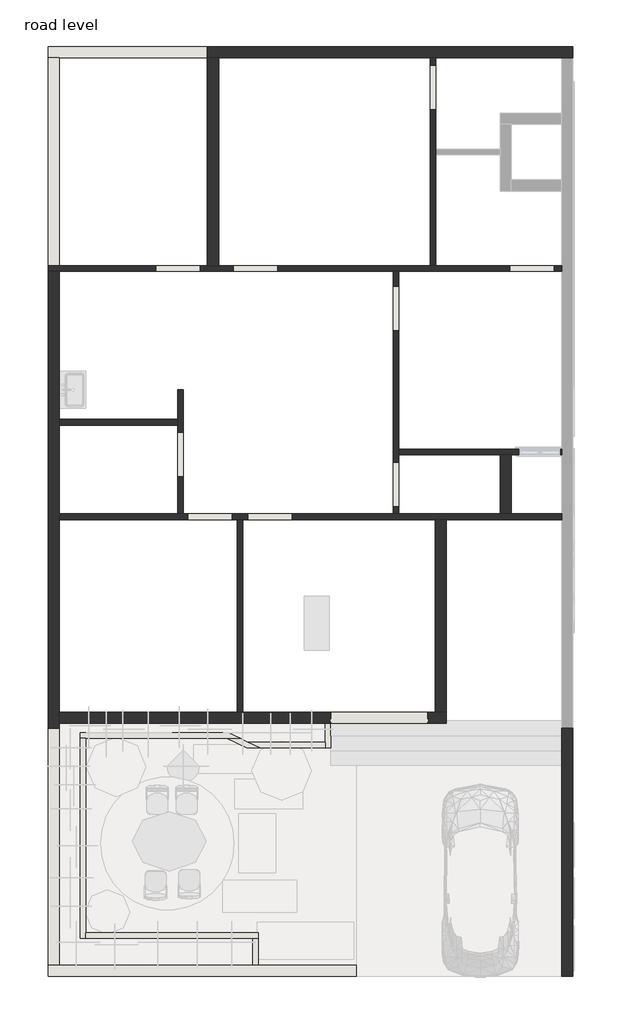
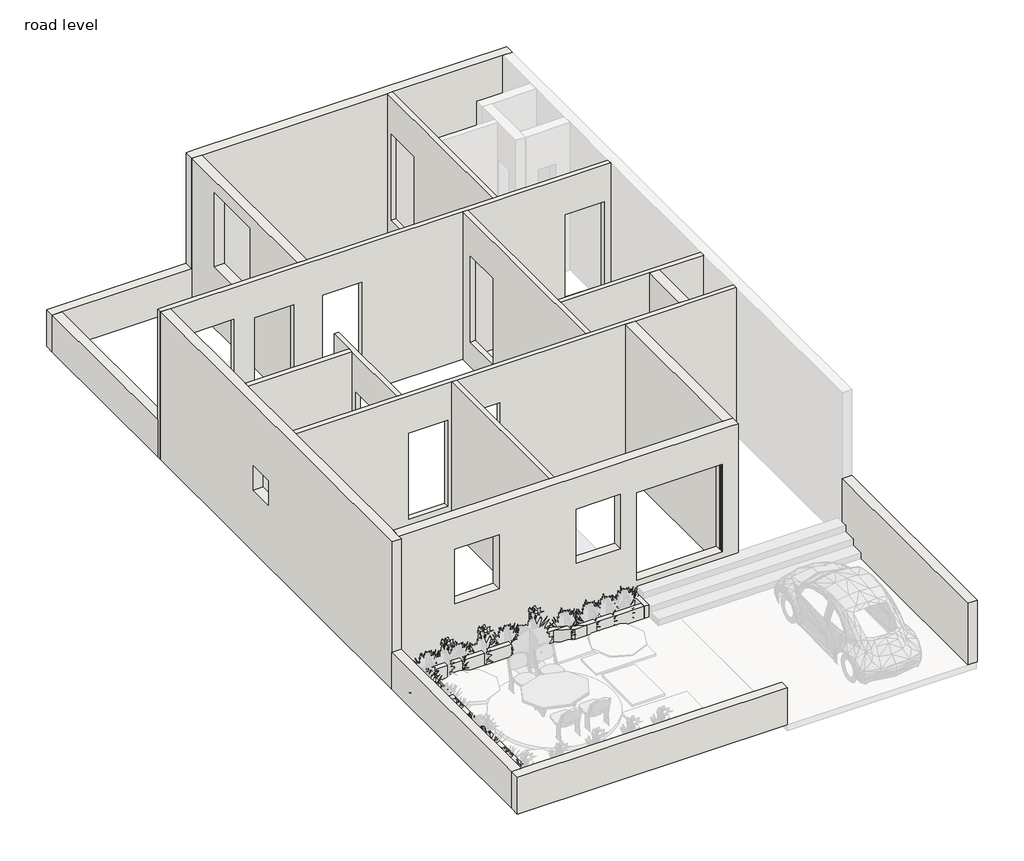
# One storey, part 1 of 2: 26 walls.
"""IFC4 building model written with IfcOpenShell, lengths in millimetres."""

from ifc_helpers import new_model, si_unit, frame, origin, origin_with_axes, place, context, project, spatial, polyline, outline, extrude, faceted_brep, element, save

model = new_model("IFC4")

# Units and contexts
model_context = context("Model", 3, world=origin())
ifc_project = project(units=[si_unit("LENGTHUNIT", "METRE", prefix="MILLI")], contexts=[model_context])

# Site, building, storey
site = spatial("IfcSite", under=ifc_project)
building = spatial("IfcBuilding", under=site)
storey = spatial("IfcBuildingStorey", under=building, Name="road level", Elevation=0.0)

# Walls
placement = place(None, origin())
element("IfcWall", 1, at=placement, inside=storey, context=model_context, shape_type="Brep", body=[
    faceted_brep([(-8110.3498597, 12578.2257925, 0.0), (-7881.7498597, 12578.2257925, 0.0), (-4833.7498597, 12578.2257925, 0.0), (-4719.4498597, 12578.2257925, 0.0), (-4719.4498597, 12578.2257925, 914.4), (-4833.7498597, 12578.2257925, 914.4), (-7881.7498597, 12578.2257925, 914.4), (-8110.3498597, 12578.2257925, 914.4), (-8110.3498597, 12806.8257925, 0.0), (-8110.3498597, 12806.8257925, 914.4), (-4833.7498597, 12806.8257925, 914.4), (-4719.4498597, 12806.8257925, 914.4), (-4719.4498597, 12806.8257925, 0.0)], [[[0, 1, 2, 3, 4, 5, 6, 7]], [[8, 9, 10, 11, 12]], [[3, 2, 1, 0, 8, 12]], [[4, 3, 12, 11]], [[7, 6, 5, 4, 11, 10, 9]], [[0, 7, 9, 8]]]),
])
element("IfcWall", 2, at=placement, inside=storey, context=model_context, shape_type="Brep", body=[
    faceted_brep([(-1774.9490674, -6090.7742075, 0.0), (-3784.6993887, -6090.7742075, 0.0), (-3898.9993887, -6090.7742075, 0.0), (-7881.7498597, -6090.7742075, 0.0), (-8110.3498597, -6090.7742075, 0.0), (-8110.3498597, -6090.7742075, 914.4), (-7881.7498597, -6090.7742075, 914.4), (-1774.9490674, -6090.7742075, 914.4), (-1774.9490674, -6319.3742075, 0.0), (-1774.9490674, -6319.3742075, 914.4), (-8110.3498597, -6319.3742075, 914.4), (-8110.3498597, -6319.3742075, 0.0)], [[[0, 1, 2, 3, 4, 5, 6, 7]], [[8, 9, 10, 11]], [[4, 3, 2, 1, 0, 8, 11]], [[7, 6, 5, 10, 9]], [[0, 7, 9, 8]], [[5, 4, 11, 10]]]),
])
element("IfcWall", 3, at=placement, inside=storey, context=model_context, shape_type="SweptSolid", body=[
    extrude(outline(polyline([(-7881.7498597, -1213.9742075), (-7881.7498597, -6090.7742075), (-8110.3498597, -6090.7742075), (-8110.3498597, -1213.9742075), (-7881.7498597, -1213.9742075)])), origin_with_axes(), (0.0, 0.0, 1.0), 914.4),
])
element("IfcWall", 4, at=placement, inside=storey, context=model_context, shape_type="Brep", body=[
    faceted_brep([(-4833.7498597, 12578.2257925, 3657.6), (-4833.7498597, 12578.2257925, 914.4), (-4833.7498597, 12578.2257925, 0.0), (-4833.7498597, 8298.3257925, 0.0), (-4833.7498597, 8298.3257925, 3657.6), (-4833.7498597, 11663.8257925, 3352.8), (-4833.7498597, 10216.0257925, 3352.8), (-4833.7498597, 10216.0257925, 1524.0), (-4833.7498597, 11663.8257925, 1524.0), (-4605.1498597, 12578.2257925, 0.0), (-4605.1498597, 12578.2257925, 3657.6), (-4605.1498597, 8298.3257925, 3657.6), (-4605.1498597, 8298.3257925, 0.0), (-4605.1498597, 11663.8257925, 3352.8), (-4605.1498597, 11663.8257925, 1524.0), (-4605.1498597, 10216.0257925, 1524.0), (-4605.1498597, 10216.0257925, 3352.8), (-4719.4498597, 12578.2257925, 0.0)], [[[0, 1, 2, 3, 4], [5, 6, 7, 8]], [[9, 10, 11, 12], [13, 14, 15, 16]], [[3, 2, 17, 9, 12]], [[14, 13, 5, 8]], [[15, 14, 8, 7]], [[16, 15, 7, 6]], [[13, 16, 6, 5]], [[0, 4, 11, 10]], [[0, 10, 9, 17, 2, 1]], [[3, 12, 11, 4]]]),
])
element("IfcWall", 5, at=placement, inside=storey, context=model_context, shape_type="Brep", body=[
    faceted_brep([(2456.0501403, 8298.3257925, 0.0), (-134.7498597, 8298.3257925, 0.0), (-249.0498597, 8298.3257925, 0.0), (-4605.1498597, 8298.3257925, 0.0), (-4833.7498597, 8298.3257925, 0.0), (-7881.7498597, 8298.3257925, 0.0), (-8110.3498597, 8298.3257925, 0.0), (-8110.3498597, 8298.3257925, 914.4), (-8110.3498597, 8298.3257925, 3200.4), (-8110.3498597, 8298.3257925, 3657.6), (-7881.7498597, 8298.3257925, 3657.6), (-4833.7498597, 8298.3257925, 3657.6), (-4605.1498597, 8298.3257925, 3657.6), (-249.0498597, 8298.3257925, 3657.6), (-134.7498597, 8298.3257925, 3657.6), (2456.0501403, 8298.3257925, 3657.6), (1389.2501403, 8298.3257925, 609.6), (2303.6501403, 8298.3257925, 609.6), (2303.6501403, 8298.3257925, 2743.2), (1389.2501403, 8298.3257925, 2743.2), (-3385.9498597, 8298.3257925, 609.6), (-3385.9498597, 8298.3257925, 2743.2), (-4300.3498597, 8298.3257925, 2743.2), (-4300.3498597, 8298.3257925, 609.6), (-5900.5498597, 8298.3257925, 609.6), (-4986.1498597, 8298.3257925, 609.6), (-4986.1498597, 8298.3257925, 2743.2), (-5900.5498597, 8298.3257925, 2743.2), (-6383.1498597, 8298.3257925, 2870.2), (-7424.5498597, 8298.3257925, 2870.2), (-7424.5498597, 8298.3257925, 1524.0), (-6383.1498597, 8298.3257925, 1524.0), (2456.0501403, 8184.0257925, 0.0), (2456.0501403, 8184.0257925, 3657.6), (-896.7498597, 8184.0257925, 3657.6), (-1011.0498597, 8184.0257925, 3657.6), (-7881.7498597, 8184.0257925, 3657.6), (-8110.3498597, 8184.0257925, 3657.6), (-8110.3498597, 8184.0257925, 3200.4), (-8110.3498597, 8184.0257925, 0.0), (-7881.7498597, 8184.0257925, 0.0), (-1011.0498597, 8184.0257925, 0.0), (-896.7498597, 8184.0257925, 0.0), (1389.2501403, 8184.0257925, 609.6), (1389.2501403, 8184.0257925, 2743.2), (2303.6501403, 8184.0257925, 2743.2), (2303.6501403, 8184.0257925, 609.6), (-3385.9498597, 8184.0257925, 609.6), (-4300.3498597, 8184.0257925, 609.6), (-4300.3498597, 8184.0257925, 2743.2), (-3385.9498597, 8184.0257925, 2743.2), (-5900.5498597, 8184.0257925, 609.6), (-5900.5498597, 8184.0257925, 2743.2), (-4986.1498597, 8184.0257925, 2743.2), (-4986.1498597, 8184.0257925, 609.6), (-6383.1498597, 8184.0257925, 2870.2), (-6383.1498597, 8184.0257925, 1524.0), (-7424.5498597, 8184.0257925, 1524.0), (-7424.5498597, 8184.0257925, 2870.2)], [[[0, 1, 2, 3, 4, 5, 6, 7, 8, 9, 10, 11, 12, 13, 14, 15], [16, 17, 18, 19], [20, 21, 22, 23], [24, 25, 26, 27], [28, 29, 30, 31]], [[32, 33, 34, 35, 36, 37, 38, 39, 40, 41, 42], [43, 44, 45, 46], [47, 48, 49, 50], [51, 52, 53, 54], [55, 56, 57, 58]], [[6, 5, 4, 3, 2, 1, 0, 32, 42, 41, 40, 39]], [[0, 15, 33, 32]], [[17, 16, 43, 46]], [[18, 17, 46, 45]], [[19, 18, 45, 44]], [[16, 19, 44, 43]], [[48, 47, 20, 23]], [[49, 48, 23, 22]], [[50, 49, 22, 21]], [[47, 50, 21, 20]], [[25, 24, 51, 54]], [[26, 25, 54, 53]], [[27, 26, 53, 52]], [[24, 27, 52, 51]], [[56, 55, 28, 31]], [[57, 56, 31, 30]], [[58, 57, 30, 29]], [[55, 58, 29, 28]], [[15, 14, 13, 12, 11, 10, 9, 37, 36, 35, 34, 33]], [[6, 39, 38, 37, 9, 8, 7]]]),
])
element("IfcWall", 6, at=placement, inside=storey, context=model_context, shape_type="Brep", body=[
    faceted_brep([(-249.0498597, 12578.2257925, 0.0), (-249.0498597, 8298.3257925, 0.0), (-249.0498597, 8298.3257925, 3657.6), (-249.0498597, 12578.2257925, 3657.6), (-249.0498597, 11511.4257925, 609.6), (-249.0498597, 12425.8257925, 609.6), (-249.0498597, 12425.8257925, 2743.2), (-249.0498597, 11511.4257925, 2743.2), (-134.7498597, 12578.2257925, 0.0), (-134.7498597, 12578.2257925, 3657.6), (-134.7498597, 10698.6257925, 3657.6), (-134.7498597, 10584.3257925, 3657.6), (-134.7498597, 8298.3257925, 3657.6), (-134.7498597, 8298.3257925, 0.0), (-134.7498597, 10584.3257925, 0.0), (-134.7498597, 10698.6257925, 0.0), (-134.7498597, 11511.4257925, 609.6), (-134.7498597, 11511.4257925, 2743.2), (-134.7498597, 12425.8257925, 2743.2), (-134.7498597, 12425.8257925, 609.6)], [[[0, 1, 2, 3], [4, 5, 6, 7]], [[8, 9, 10, 11, 12, 13, 14, 15], [16, 17, 18, 19]], [[1, 0, 8, 15, 14, 13]], [[0, 3, 9, 8]], [[5, 4, 16, 19]], [[6, 5, 19, 18]], [[7, 6, 18, 17]], [[4, 7, 17, 16]], [[3, 2, 12, 11, 10, 9]], [[1, 13, 12, 2]]]),
])
element("IfcWall", 7, at=placement, inside=storey, context=model_context, shape_type="SweptSolid", body=[
    extrude(outline(polyline([(-5443.3498597, 5021.7257925), (-7881.7498597, 5021.7257925), (-7881.7498597, 5136.0257925), (-5443.3498597, 5136.0257925), (-5443.3498597, 5021.7257925)])), origin_with_axes(), (0.0, 0.0, 1.0), 3657.6),
])
element("IfcWall", 8, at=placement, inside=storey, context=model_context, shape_type="Brep", body=[
    faceted_brep([(-5329.0498597, 3192.9257925, 3657.6), (-5329.0498597, 3192.9257925, 0.0), (-5329.0498597, 5745.6257925, 0.0), (-5329.0498597, 5745.6257925, 3657.6), (-5329.0498597, 3954.9257925, 609.6), (-5329.0498597, 3954.9257925, 2743.2), (-5329.0498597, 4869.3257925, 2743.2), (-5329.0498597, 4869.3257925, 609.6), (-5443.3498597, 3192.9257925, 0.0), (-5443.3498597, 3192.9257925, 3657.6), (-5443.3498597, 5021.7257925, 3657.6), (-5443.3498597, 5136.0257925, 3657.6), (-5443.3498597, 5745.6257925, 3657.6), (-5443.3498597, 5745.6257925, 0.0), (-5443.3498597, 5136.0257925, 0.0), (-5443.3498597, 5021.7257925, 0.0), (-5443.3498597, 3954.9257925, 609.6), (-5443.3498597, 4869.3257925, 609.6), (-5443.3498597, 4869.3257925, 2743.2), (-5443.3498597, 3954.9257925, 2743.2)], [[[0, 1, 2, 3], [4, 5, 6, 7]], [[8, 9, 10, 11, 12, 13, 14, 15], [16, 17, 18, 19]], [[2, 1, 8, 15, 14, 13]], [[3, 2, 13, 12]], [[17, 16, 4, 7]], [[18, 17, 7, 6]], [[19, 18, 6, 5]], [[16, 19, 5, 4]], [[0, 3, 12, 11, 10, 9]], [[0, 9, 8, 1]]]),
])
element("IfcWall", 9, at=placement, inside=storey, context=model_context, shape_type="Brep", body=[
    faceted_brep([(-7881.7498597, 3078.6257925, 3657.6), (-7881.7498597, 3078.6257925, 0.0), (-4224.1498597, 3078.6257925, 0.0), (-4109.8498597, 3078.6257925, 0.0), (-147.4498597, 3078.6257925, 0.0), (81.1501403, 3078.6257925, 0.0), (2456.0501403, 3078.6257925, 0.0), (2456.0501403, 3078.6257925, 3657.6), (2430.6501403, 3078.6257925, 3657.6), (81.1501403, 3078.6257925, 3657.6), (-147.4498597, 3078.6257925, 3657.6), (-4109.8498597, 3078.6257925, 3657.6), (-4224.1498597, 3078.6257925, 3657.6), (-5233.7998597, 3078.6257925, 609.6), (-5233.7998597, 3078.6257925, 2743.2), (-4319.3998597, 3078.6257925, 2743.2), (-4319.3998597, 3078.6257925, 609.6), (-3093.8498597, 3078.6257925, 609.6), (-4008.2498597, 3078.6257925, 609.6), (-4008.2498597, 3078.6257925, 2743.2), (-3093.8498597, 3078.6257925, 2743.2), (-7881.7498597, 3192.9257925, 0.0), (-7881.7498597, 3192.9257925, 3657.6), (-5443.3498597, 3192.9257925, 3657.6), (-5329.0498597, 3192.9257925, 3657.6), (-1011.0498597, 3192.9257925, 3657.6), (-896.7498597, 3192.9257925, 3657.6), (1186.0501403, 3192.9257925, 3657.6), (1414.6501403, 3192.9257925, 3657.6), (2456.0501403, 3192.9257925, 3657.6), (2456.0501403, 3192.9257925, 0.0), (1414.6501403, 3192.9257925, 0.0), (1186.0501403, 3192.9257925, 0.0), (-896.7498597, 3192.9257925, 0.0), (-1011.0498597, 3192.9257925, 0.0), (-5329.0498597, 3192.9257925, 0.0), (-5443.3498597, 3192.9257925, 0.0), (-5233.7998597, 3192.9257925, 609.6), (-4319.3998597, 3192.9257925, 609.6), (-4319.3998597, 3192.9257925, 2743.2), (-5233.7998597, 3192.9257925, 2743.2), (-3093.8498597, 3192.9257925, 609.6), (-3093.8498597, 3192.9257925, 2743.2), (-4008.2498597, 3192.9257925, 2743.2), (-4008.2498597, 3192.9257925, 609.6)], [[[0, 1, 2, 3, 4, 5, 6, 7, 8, 9, 10, 11, 12], [13, 14, 15, 16], [17, 18, 19, 20]], [[21, 22, 23, 24, 25, 26, 27, 28, 29, 30, 31, 32, 33, 34, 35, 36], [37, 38, 39, 40], [41, 42, 43, 44]], [[6, 5, 4, 3, 2, 1, 21, 36, 35, 34, 33, 32, 31, 30]], [[7, 6, 30, 29]], [[38, 37, 13, 16]], [[39, 38, 16, 15]], [[40, 39, 15, 14]], [[37, 40, 14, 13]], [[18, 17, 41, 44]], [[19, 18, 44, 43]], [[20, 19, 43, 42]], [[17, 20, 42, 41]], [[0, 12, 11, 10, 9, 8, 7, 29, 28, 27, 26, 25, 24, 23, 22]], [[0, 22, 21, 1]]]),
])
element("IfcWall", 10, at=placement, inside=storey, context=model_context, shape_type="Brep", body=[
    faceted_brep([(-7881.7498597, -1112.3742075, 0.0), (-2415.5726479, -1112.3742075, 0.0), (-2301.2726479, -1112.3742075, 0.0), (81.1501403, -1112.3742075, 0.0), (81.1501403, -1112.3742075, 3657.6), (-147.4498597, -1112.3742075, 3657.6), (-7881.7498597, -1112.3742075, 3657.6), (-2299.8498597, -1112.3742075, 2779.1), (-299.8498597, -1112.3742075, 2779.1), (-299.8498597, -1112.3742075, 609.6), (-2299.8498597, -1112.3742075, 609.6), (-6573.6498597, -1112.3742075, 1524.0), (-6573.6498597, -1112.3742075, 2870.2), (-5532.2498597, -1112.3742075, 2870.2), (-5532.2498597, -1112.3742075, 1524.0), (-3725.5498597, -1112.3742075, 1524.0), (-3725.5498597, -1112.3742075, 2870.2), (-2684.1498597, -1112.3742075, 2870.2), (-2684.1498597, -1112.3742075, 1524.0), (81.1501403, -883.7742075, 0.0), (-147.4498597, -883.7742075, 0.0), (-4109.8498597, -883.7742075, 0.0), (-4224.1498597, -883.7742075, 0.0), (-7881.7498597, -883.7742075, 0.0), (-7881.7498597, -883.7742075, 3657.6), (-4224.1498597, -883.7742075, 3657.6), (-4109.8498597, -883.7742075, 3657.6), (-147.4498597, -883.7742075, 3657.6), (81.1501403, -883.7742075, 3657.6), (81.1501403, -883.7742075, 3200.4), (-299.8498597, -883.7742075, 2779.1), (-2299.8498597, -883.7742075, 2779.1), (-2299.8498597, -883.7742075, 609.6), (-299.8498597, -883.7742075, 609.6), (-6573.6498597, -883.7742075, 2870.2), (-6573.6498597, -883.7742075, 1524.0), (-5532.2498597, -883.7742075, 1524.0), (-5532.2498597, -883.7742075, 2870.2), (-3725.5498597, -883.7742075, 2870.2), (-3725.5498597, -883.7742075, 1524.0), (-2684.1498597, -883.7742075, 1524.0), (-2684.1498597, -883.7742075, 2870.2), (-2299.8498597, -1092.3742075, 2779.1), (-299.8498597, -1092.3742075, 2779.1), (-299.8498597, -1022.3742075, 2779.1), (-2299.8498597, -1022.3742075, 2779.1), (-2299.8498597, -1022.3742075, 609.6), (-2314.8498597, -1022.3742075, 609.6), (-2314.8498597, -1092.3742075, 609.6), (-2299.8498597, -1092.3742075, 609.6), (-299.8498597, -1092.3742075, 609.6), (-284.8498597, -1092.3742075, 609.6), (-284.8498597, -1022.3742075, 609.6), (-299.8498597, -1022.3742075, 609.6), (-284.8498597, -1022.3742075, 2794.1), (-2314.8498597, -1022.3742075, 2794.1), (-2314.8498597, -1092.3742075, 2794.1), (-284.8498597, -1092.3742075, 2794.1)], [[[0, 1, 2, 3, 4, 5, 6], [7, 8, 9, 10], [11, 12, 13, 14], [15, 16, 17, 18]], [[19, 20, 21, 22, 23, 24, 25, 26, 27, 28, 29], [30, 31, 32, 33], [34, 35, 36, 37], [38, 39, 40, 41]], [[3, 2, 1, 0, 23, 22, 21, 20, 19]], [[42, 43, 8, 7]], [[44, 45, 31, 30]], [[46, 47, 48, 49, 10, 9, 50, 51, 52, 53, 33, 32]], [[53, 44, 30, 33]], [[45, 46, 32, 31]], [[45, 44, 53, 52, 54, 55, 47, 46]], [[48, 47, 55, 56]], [[43, 42, 49, 48, 56, 57, 51, 50]], [[49, 42, 7, 10]], [[43, 50, 9, 8]], [[52, 51, 57, 54]], [[55, 54, 57, 56]], [[35, 34, 12, 11]], [[36, 35, 11, 14]], [[37, 36, 14, 13]], [[34, 37, 13, 12]], [[39, 38, 16, 15]], [[40, 39, 15, 18]], [[41, 40, 18, 17]], [[38, 41, 17, 16]], [[3, 19, 29, 28, 4]], [[6, 5, 4, 28, 27, 26, 25, 24]], [[23, 0, 6, 24]]]),
])
element("IfcWall", 11, at=placement, inside=storey, context=model_context, shape_type="SweptSolid", body=[
    extrude(outline(polyline([(-4109.8498597, 3078.6257925), (-4109.8498597, -883.7742075), (-4224.1498597, -883.7742075), (-4224.1498597, 3078.6257925), (-4109.8498597, 3078.6257925)])), origin_with_axes(), (0.0, 0.0, 1.0), 3657.6),
])
element("IfcWall", 12, at=placement, inside=storey, context=model_context, shape_type="Brep", body=[
    faceted_brep([(81.1501403, -883.7742075, 3657.6), (81.1501403, -883.7742075, 0.0), (81.1501403, 3078.6257925, 0.0), (81.1501403, 3078.6257925, 3657.6), (81.1501403, 157.6257925, 3657.6), (-147.4498597, -883.7742075, 0.0), (-147.4498597, -883.7742075, 3657.6), (-147.4498597, 3078.6257925, 3657.6), (-147.4498597, 3078.6257925, 0.0)], [[[0, 1, 2, 3, 4]], [[5, 6, 7, 8]], [[2, 1, 5, 8]], [[0, 4, 3, 7, 6]], [[0, 6, 5, 1]], [[2, 8, 7, 3]]]),
])
element("IfcWall", 13, at=placement, inside=storey, context=model_context, shape_type="Brep", body=[
    faceted_brep([(2456.0501403, 4526.4257925, 0.0), (-896.7498597, 4526.4257925, 0.0), (-896.7498597, 4526.4257925, 3657.6), (2456.0501403, 4526.4257925, 3657.6), (2430.6501403, 4526.4257925, 1828.8), (1567.0501403, 4526.4257925, 1828.8), (1567.0501403, 4526.4257925, 914.4), (2430.6501403, 4526.4257925, 914.4), (2456.0501403, 4412.1257925, 0.0), (2456.0501403, 4412.1257925, 3657.6), (1414.6501403, 4412.1257925, 3657.6), (1186.0501403, 4412.1257925, 3657.6), (-896.7498597, 4412.1257925, 3657.6), (-896.7498597, 4412.1257925, 0.0), (1186.0501403, 4412.1257925, 0.0), (1414.6501403, 4412.1257925, 0.0), (2430.6501403, 4412.1257925, 1828.8), (2430.6501403, 4412.1257925, 914.4), (1567.0501403, 4412.1257925, 914.4), (1567.0501403, 4412.1257925, 1828.8)], [[[0, 1, 2, 3], [4, 5, 6, 7]], [[8, 9, 10, 11, 12, 13, 14, 15], [16, 17, 18, 19]], [[1, 0, 8, 15, 14, 13]], [[0, 3, 9, 8]], [[17, 16, 4, 7]], [[18, 17, 7, 6]], [[19, 18, 6, 5]], [[16, 19, 5, 4]], [[3, 2, 12, 11, 10, 9]], [[1, 13, 12, 2]]]),
])
element("IfcWall", 14, at=placement, inside=storey, context=model_context, shape_type="SweptSolid", body=[
    extrude(outline(polyline([(3192.9257925, 0.0), (3192.9257925, 3657.6), (4412.1257925, 3657.6), (4412.1257925, 0.0), (3192.9257925, 0.0)]), holes=[polyline([(3599.3257925, 2133.6), (3599.3257925, 1524.0), (4005.7257925, 1524.0), (4005.7257925, 2133.6), (3599.3257925, 2133.6)])]), frame((1186.0501403, 0.0, 0.0), z_axis=(1.0, 0.0, 0.0), x_axis=(0.0, 1.0, 0.0)), (0.0, 0.0, 1.0), 228.6),
])
element("IfcWall", 15, at=placement, inside=storey, context=model_context, shape_type="Brep", body=[
    faceted_brep([(-896.7498597, 3192.9257925, 3657.6), (-896.7498597, 3192.9257925, 0.0), (-896.7498597, 4412.1257925, 0.0), (-896.7498597, 4526.4257925, 0.0), (-896.7498597, 8184.0257925, 0.0), (-896.7498597, 8184.0257925, 3657.6), (-896.7498597, 4526.4257925, 3657.6), (-896.7498597, 4412.1257925, 3657.6), (-896.7498597, 6964.8257925, 609.6), (-896.7498597, 6964.8257925, 2743.2), (-896.7498597, 7879.2257925, 2743.2), (-896.7498597, 7879.2257925, 609.6), (-896.7498597, 4259.7257925, 609.6), (-896.7498597, 3345.3257925, 609.6), (-896.7498597, 3345.3257925, 2743.2), (-896.7498597, 4259.7257925, 2743.2), (-1011.0498597, 3192.9257925, 0.0), (-1011.0498597, 3192.9257925, 3657.6), (-1011.0498597, 8184.0257925, 3657.6), (-1011.0498597, 8184.0257925, 0.0), (-1011.0498597, 6964.8257925, 609.6), (-1011.0498597, 7879.2257925, 609.6), (-1011.0498597, 7879.2257925, 2743.2), (-1011.0498597, 6964.8257925, 2743.2), (-1011.0498597, 4259.7257925, 609.6), (-1011.0498597, 4259.7257925, 2743.2), (-1011.0498597, 3345.3257925, 2743.2), (-1011.0498597, 3345.3257925, 609.6)], [[[0, 1, 2, 3, 4, 5, 6, 7], [8, 9, 10, 11], [12, 13, 14, 15]], [[16, 17, 18, 19], [20, 21, 22, 23], [24, 25, 26, 27]], [[4, 3, 2, 1, 16, 19]], [[21, 20, 8, 11]], [[22, 21, 11, 10]], [[23, 22, 10, 9]], [[20, 23, 9, 8]], [[13, 12, 24, 27]], [[14, 13, 27, 26]], [[15, 14, 26, 25]], [[12, 15, 25, 24]], [[0, 7, 6, 5, 18, 17]], [[4, 19, 18, 5]], [[0, 17, 16, 1]]]),
])
element("IfcWall", 16, at=placement, inside=storey, context=model_context, shape_type="Brep", body=[
    faceted_brep([(-7881.7498597, -1213.9742075, 0.0), (-7881.7498597, -1112.3742075, 0.0), (-7881.7498597, -883.7742075, 0.0), (-7881.7498597, 3078.6257925, 0.0), (-7881.7498597, 3192.9257925, 0.0), (-7881.7498597, 5021.7257925, 0.0), (-7881.7498597, 5136.0257925, 0.0), (-7881.7498597, 8184.0257925, 0.0), (-7881.7498597, 8184.0257925, 3657.6), (-7881.7498597, 5136.0257925, 3657.6), (-7881.7498597, 5021.7257925, 3657.6), (-7881.7498597, 3192.9257925, 3657.6), (-7881.7498597, 3078.6257925, 3657.6), (-7881.7498597, -883.7742075, 3657.6), (-7881.7498597, -1112.3742075, 3657.6), (-7881.7498597, -1213.9742075, 3657.6), (-7881.7498597, -1213.9742075, 914.4), (-7881.7498597, 4412.1257925, 2133.6), (-7881.7498597, 4412.1257925, 1524.0), (-7881.7498597, 3802.5257925, 1524.0), (-7881.7498597, 3802.5257925, 2133.6), (-8110.3498597, -1213.9742075, 0.0), (-8110.3498597, -1213.9742075, 914.4), (-8110.3498597, -1213.9742075, 3657.6), (-8110.3498597, 8184.0257925, 3657.6), (-8110.3498597, 8184.0257925, 0.0), (-8110.3498597, 4412.1257925, 2133.6), (-8110.3498597, 3802.5257925, 2133.6), (-8110.3498597, 3802.5257925, 1524.0), (-8110.3498597, 4412.1257925, 1524.0)], [[[0, 1, 2, 3, 4, 5, 6, 7, 8, 9, 10, 11, 12, 13, 14, 15, 16], [17, 18, 19, 20]], [[21, 22, 23, 24, 25], [26, 27, 28, 29]], [[7, 6, 5, 4, 3, 2, 1, 0, 21, 25]], [[0, 16, 15, 23, 22, 21]], [[17, 20, 27, 26]], [[20, 19, 28, 27]], [[19, 18, 29, 28]], [[18, 17, 26, 29]], [[15, 14, 13, 12, 11, 10, 9, 8, 24, 23]], [[7, 25, 24, 8]]]),
])
element("IfcWall", 17, at=placement, inside=storey, context=model_context, shape_type="SweptSolid", body=[
    extrude(outline(polyline([(-7881.7498597, 12578.2257925), (-7881.7498597, 8298.3257925), (-8110.3498597, 8298.3257925), (-8110.3498597, 12578.2257925), (-7881.7498597, 12578.2257925)])), origin_with_axes(), (0.0, 0.0, 1.0), 914.4),
])
element("IfcWall", 18, at=placement, inside=storey, context=model_context, shape_type="Brep", body=[
    faceted_brep([(-4719.4498597, 12578.2257925, 0.0), (-4605.1498597, 12578.2257925, 0.0), (-249.0498597, 12578.2257925, 0.0), (-134.7498597, 12578.2257925, 0.0), (2456.0501403, 12578.2257925, 0.0), (2684.6501403, 12578.2257925, 0.0), (2684.6501403, 12578.2257925, 3657.6), (2456.0501403, 12578.2257925, 3657.6), (-134.7498597, 12578.2257925, 3657.6), (-249.0498597, 12578.2257925, 3657.6), (-4605.1498597, 12578.2257925, 3657.6), (-4833.7498597, 12578.2257925, 3657.6), (-4833.7498597, 12578.2257925, 3200.4), (-4833.7498597, 12578.2257925, 914.4), (-4719.4498597, 12578.2257925, 914.4), (-4719.4498597, 12806.8257925, 0.0), (-4719.4498597, 12806.8257925, 914.4), (-4833.7498597, 12806.8257925, 914.4), (-4833.7498597, 12806.8257925, 3200.4), (-4833.7498597, 12806.8257925, 3657.6), (-4605.1498597, 12806.8257925, 3657.6), (2684.6501403, 12806.8257925, 3657.6), (2684.6501403, 12806.8257925, 0.0)], [[[0, 1, 2, 3, 4, 5, 6, 7, 8, 9, 10, 11, 12, 13, 14]], [[15, 16, 17, 18, 19, 20, 21, 22]], [[5, 4, 3, 2, 1, 0, 15, 22]], [[6, 5, 22, 21]], [[0, 14, 16, 15]], [[13, 17, 16, 14]], [[11, 10, 9, 8, 7, 6, 21, 20, 19]], [[11, 19, 18, 17, 13, 12]]]),
])
element("IfcWall", 19, at=placement, inside=storey, context=model_context, shape_type="SweptSolid", body=[
    extrude(outline(polyline([(2456.0501403, -6319.3742075), (2456.0501403, -1213.9742075), (2684.6501403, -1213.9742075), (2684.6501403, -6319.3742075), (2456.0501403, -6319.3742075)])), origin_with_axes(), (0.0, 0.0, 1.0), 1524.0),
])
element("IfcWall", 20, at=placement, inside=storey, context=model_context, shape_type="Brep", body=[
    faceted_brep([(-7454.9993887, -1423.8266914, 0.0), (-7340.6993887, -1423.8266914, 0.0), (-4432.3390886, -1423.8266914, 0.0), (-4161.8822477, -1423.8266914, 0.0), (-4161.8822477, -1423.8266914, 304.8), (-4432.3390886, -1423.8266914, 304.8), (-7340.6993887, -1423.8266914, 304.8), (-7454.9993887, -1423.8266914, 304.8), (-7454.9993887, -1309.5266914, 0.0), (-7454.9993887, -1309.5266914, 304.8), (-4406.9993887, -1309.5266914, 304.8), (-4406.9993887, -1309.5266914, 0.0)], [[[0, 1, 2, 3, 4, 5, 6, 7]], [[8, 9, 10, 11]], [[3, 2, 1, 0, 8, 11]], [[7, 6, 5, 4, 10, 9]], [[4, 3, 11, 10]], [[0, 7, 9, 8]]]),
])
element("IfcWall", 21, at=placement, inside=storey, context=model_context, shape_type="Brep", body=[
    faceted_brep([(-4432.3390886, -1423.8266914, 0.0), (-4028.4424978, -1612.1667647, 0.0), (-4028.4424978, -1612.1667647, 304.8), (-4432.3390886, -1423.8266914, 304.8), (-4161.8822477, -1423.8266914, 0.0), (-4161.8822477, -1423.8266914, 304.8), (-4003.1027979, -1497.8667647, 304.8), (-3757.9856569, -1612.1667647, 304.8), (-3757.9856569, -1612.1667647, 0.0), (-4003.1027979, -1497.8667647, 0.0)], [[[0, 1, 2, 3]], [[4, 5, 6, 7, 8, 9]], [[1, 0, 4, 9, 8]], [[3, 2, 7, 6, 5]], [[0, 3, 5, 4]], [[2, 1, 8, 7]]]),
])
element("IfcWall", 22, at=placement, inside=storey, context=model_context, shape_type="SweptSolid", body=[
    extrude(outline(polyline([(-2415.5726479, -1612.1667647), (-3757.9856569, -1612.1667647), (-4003.1027979, -1497.8667647), (-2415.5726479, -1497.8667647), (-2415.5726479, -1612.1667647)])), origin_with_axes(), (0.0, 0.0, 1.0), 304.8),
])
element("IfcWall", 23, at=placement, inside=storey, context=model_context, shape_type="Brep", body=[
    faceted_brep([(-2301.2726479, -1612.1667647, 0.0), (-2301.2726479, -1112.3742075, 0.0), (-2301.2726479, -1112.3742075, 304.8), (-2301.2726479, -1612.1667647, 304.8), (-2415.5726479, -1612.1667647, 0.0), (-2415.5726479, -1612.1667647, 304.8), (-2415.5726479, -1497.8667647, 304.8), (-2415.5726479, -1112.3742075, 304.8), (-2415.5726479, -1112.3742075, 0.0), (-2415.5726479, -1497.8667647, 0.0)], [[[0, 1, 2, 3]], [[4, 5, 6, 7, 8, 9]], [[1, 0, 4, 9, 8]], [[3, 2, 7, 6, 5]], [[0, 3, 5, 4]], [[2, 1, 8, 7]]]),
])
element("IfcWall", 24, at=placement, inside=storey, context=model_context, shape_type="Brep", body=[
    faceted_brep([(-7454.9993887, -1423.8266914, 0.0), (-7454.9993887, -5536.0025668, 0.0), (-7454.9993887, -5536.0025668, 304.8), (-7454.9993887, -1423.8266914, 304.8), (-7340.6993887, -1423.8266914, 0.0), (-7340.6993887, -1423.8266914, 304.8), (-7340.6993887, -5421.7025668, 304.8), (-7340.6993887, -5536.0025668, 304.8), (-7340.6993887, -5536.0025668, 0.0), (-7340.6993887, -5421.7025668, 0.0)], [[[0, 1, 2, 3]], [[4, 5, 6, 7, 8, 9]], [[1, 0, 4, 9, 8]], [[3, 2, 7, 6, 5]], [[0, 3, 5, 4]], [[2, 1, 8, 7]]]),
])
element("IfcWall", 25, at=placement, inside=storey, context=model_context, shape_type="Brep", body=[
    faceted_brep([(-7340.6993887, -5536.0025668, 0.0), (-3898.9993887, -5536.0025668, 0.0), (-3784.6993887, -5536.0025668, 0.0), (-3784.6993887, -5536.0025668, 304.8), (-3898.9993887, -5536.0025668, 304.8), (-7340.6993887, -5536.0025668, 304.8), (-7340.6993887, -5421.7025668, 0.0), (-7340.6993887, -5421.7025668, 304.8), (-3784.6993887, -5421.7025668, 304.8), (-3784.6993887, -5421.7025668, 0.0)], [[[0, 1, 2, 3, 4, 5]], [[6, 7, 8, 9]], [[2, 1, 0, 6, 9]], [[5, 4, 3, 8, 7]], [[0, 5, 7, 6]], [[3, 2, 9, 8]]]),
])
element("IfcWall", 26, at=placement, inside=storey, context=model_context, shape_type="SweptSolid", body=[
    extrude(outline(polyline([(-3898.9993887, -6090.7742075), (-3898.9993887, -5536.0025668), (-3784.6993887, -5536.0025668), (-3784.6993887, -6090.7742075), (-3898.9993887, -6090.7742075)])), origin_with_axes(), (0.0, 0.0, 1.0), 304.8),
])

save(model, "model.ifc")

# Revit data of these elements
# Type
#   Assembly Code = "B2010"
#   Layers, outside or top first: 0' - 9" no material (function 1)
# Type
#   Assembly Code = "B2010"
#   Layers, outside or top first: 0' - 4 1/2" no material (function 1)
# Elements 1, 2, 3, 17 (IfcWall)
#   Top Offset = 0' - 0"
#   Base Offset = 0' - 0"
#   Unconnected Height = 3' - 0"
#   wall height = 3' - 0"
#   Phase Created = New Construction
#   Base Constraint = road level
#   Materials on its faces: "Default Wall"
# Elements 4, 5, 6, 7, 8, 9, 10, 11, 12, 13, 14, 15, 16, 18 (IfcWall)
#   Top Offset = 0' - 0"
#   Base Offset = 0' - 0"
#   wall height = 12' - 0"
#   Phase Created = New Construction
#   Base Constraint = road level
#   Top Constraint = 1st floor
#   Materials on its faces: "Default Wall"
# Element 19 (IfcWall)
#   Top Offset = 0' - 0"
#   Base Offset = 0' - 0"
#   Unconnected Height = 5' - 0"
#   wall height = 5' - 0"
#   Phase Created = New Construction
#   Base Constraint = road level
#   Materials on its faces: "Default Wall"
# Elements 20, 21, 22, 23, 24, 25, 26 (IfcWall)
#   Top Offset = 0' - 0"
#   Base Offset = 0' - 0"
#   Unconnected Height = 1' - 0"
#   wall height = 1' - 0"
#   Phase Created = New Construction
#   Base Constraint = road level
#   Materials on its faces: "Default Wall"
# Materials
#   "Default Wall": colour RGB 128 128 128, transparency 0, Cost = 0
